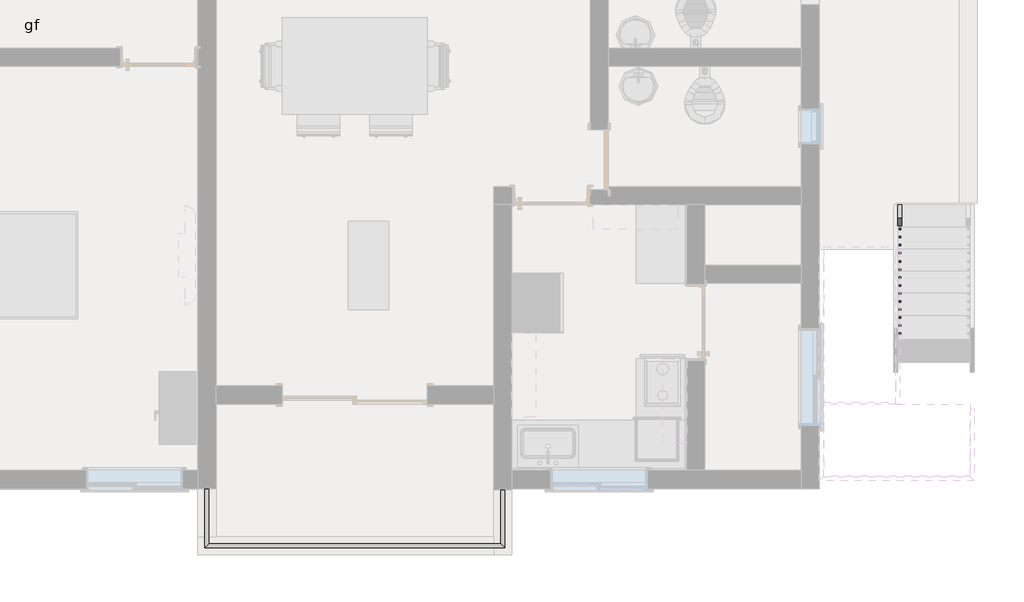
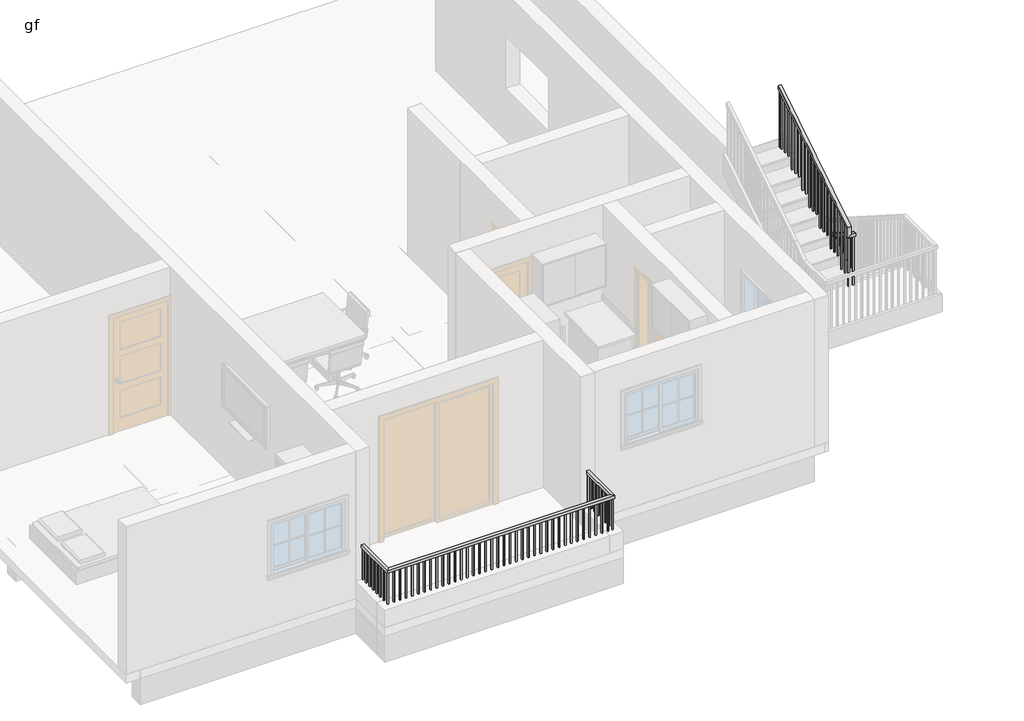
# One storey, part 4 of 8: 2 railings.
"""IFC4 building model written with IfcOpenShell, lengths in millimetres."""

from ifc_helpers import new_model, si_unit, frame, origin, place, context, project, spatial, polyline, outline, extrude, faceted_brep, element, save

model = new_model("IFC4")

# Units and contexts
model_context = context("Model", 3, world=origin())
ifc_project = project(units=[si_unit("LENGTHUNIT", "METRE", prefix="MILLI")], contexts=[model_context])

# Site, building, storey
site = spatial("IfcSite", under=ifc_project)
building = spatial("IfcBuilding", under=site)
storey = spatial("IfcBuildingStorey", under=building, Name="gf", Elevation=609.6)

# Railings
placement = place(None, origin())
element("IfcRailing", 1, ObjectType="Handrail - Rectangular", at=placement, inside=storey, context=model_context, shape_type="SolidModel", body=[
    faceted_brep([(-12350.8993763, -4611.6564015, 1524.0), (-12350.8993763, -4611.6564015, 1473.2), (-12401.6993763, -4611.6564015, 1473.2), (-12401.6993763, -4611.6564015, 1524.0), (-12350.8993763, -5303.8064015, 1524.0), (-12350.8993763, -5303.8064015, 1473.2), (-12401.6993763, -5354.6064015, 1473.2), (-12401.6993763, -5354.6064015, 1524.0), (-8667.8993763, -5303.8064015, 1524.0), (-8667.8993763, -5303.8064015, 1473.2), (-8617.0993763, -5354.6064015, 1473.2), (-8617.0993763, -5354.6064015, 1524.0), (-8667.8993763, -4618.0064015, 1524.0), (-8617.0993763, -4618.0064015, 1524.0), (-8617.0993763, -4618.0064015, 1473.2), (-8667.8993763, -4618.0064015, 1473.2)], [[[0, 1, 2, 3]], [[1, 0, 4, 5]], [[2, 1, 5, 6]], [[3, 2, 6, 7]], [[0, 3, 7, 4]], [[5, 4, 8, 9]], [[6, 5, 9, 10]], [[7, 6, 10, 11]], [[4, 7, 11, 8]], [[12, 13, 14, 15]], [[9, 8, 12, 15]], [[10, 9, 15, 14]], [[11, 10, 14, 13]], [[8, 11, 13, 12]]]),
    extrude(outline(polyline([(-8632.9743763, -4729.1314015), (-8652.0243763, -4729.1314015), (-8652.0243763, -4710.0814015), (-8632.9743763, -4710.0814015), (-8632.9743763, -4729.1314015)])), frame((0.0, 0.0, 609.6), z_axis=(0.0, 0.0, 1.0), x_axis=(1.0, 0.0, 0.0)), (0.0, 0.0, 1.0), 863.6),
    extrude(outline(polyline([(-8632.9743763, -4830.7314015), (-8652.0243763, -4830.7314015), (-8652.0243763, -4811.6814015), (-8632.9743763, -4811.6814015), (-8632.9743763, -4830.7314015)])), frame((0.0, 0.0, 609.6), z_axis=(0.0, 0.0, 1.0), x_axis=(1.0, 0.0, 0.0)), (0.0, 0.0, 1.0), 863.6),
    extrude(outline(polyline([(-8632.9743763, -4932.3314015), (-8652.0243763, -4932.3314015), (-8652.0243763, -4913.2814015), (-8632.9743763, -4913.2814015), (-8632.9743763, -4932.3314015)])), frame((0.0, 0.0, 609.6), z_axis=(0.0, 0.0, 1.0), x_axis=(1.0, 0.0, 0.0)), (0.0, 0.0, 1.0), 863.6),
    extrude(outline(polyline([(-8632.9743763, -5033.9314015), (-8652.0243763, -5033.9314015), (-8652.0243763, -5014.8814015), (-8632.9743763, -5014.8814015), (-8632.9743763, -5033.9314015)])), frame((0.0, 0.0, 609.6), z_axis=(0.0, 0.0, 1.0), x_axis=(1.0, 0.0, 0.0)), (0.0, 0.0, 1.0), 863.6),
    extrude(outline(polyline([(-8632.9743763, -5135.5314015), (-8652.0243763, -5135.5314015), (-8652.0243763, -5116.4814015), (-8632.9743763, -5116.4814015), (-8632.9743763, -5135.5314015)])), frame((0.0, 0.0, 609.6), z_axis=(0.0, 0.0, 1.0), x_axis=(1.0, 0.0, 0.0)), (0.0, 0.0, 1.0), 863.6),
    extrude(outline(polyline([(-8632.9743763, -5237.1314015), (-8652.0243763, -5237.1314015), (-8652.0243763, -5218.0814015), (-8632.9743763, -5218.0814015), (-8632.9743763, -5237.1314015)])), frame((0.0, 0.0, 609.6), z_axis=(0.0, 0.0, 1.0), x_axis=(1.0, 0.0, 0.0)), (0.0, 0.0, 1.0), 863.6),
    extrude(outline(polyline([(-8728.2243763, -5338.7314015), (-8728.2243763, -5319.6814015), (-8709.1743763, -5319.6814015), (-8709.1743763, -5338.7314015), (-8728.2243763, -5338.7314015)])), frame((0.0, 0.0, 609.6), z_axis=(0.0, 0.0, 1.0), x_axis=(1.0, 0.0, 0.0)), (0.0, 0.0, 1.0), 863.6),
    extrude(outline(polyline([(-8829.8243763, -5338.7314015), (-8829.8243763, -5319.6814015), (-8810.7743763, -5319.6814015), (-8810.7743763, -5338.7314015), (-8829.8243763, -5338.7314015)])), frame((0.0, 0.0, 609.6), z_axis=(0.0, 0.0, 1.0), x_axis=(1.0, 0.0, 0.0)), (0.0, 0.0, 1.0), 863.6),
    extrude(outline(polyline([(-8931.4243763, -5338.7314015), (-8931.4243763, -5319.6814015), (-8912.3743763, -5319.6814015), (-8912.3743763, -5338.7314015), (-8931.4243763, -5338.7314015)])), frame((0.0, 0.0, 609.6), z_axis=(0.0, 0.0, 1.0), x_axis=(1.0, 0.0, 0.0)), (0.0, 0.0, 1.0), 863.6),
    extrude(outline(polyline([(-9033.0243763, -5338.7314015), (-9033.0243763, -5319.6814015), (-9013.9743763, -5319.6814015), (-9013.9743763, -5338.7314015), (-9033.0243763, -5338.7314015)])), frame((0.0, 0.0, 609.6), z_axis=(0.0, 0.0, 1.0), x_axis=(1.0, 0.0, 0.0)), (0.0, 0.0, 1.0), 863.6),
    extrude(outline(polyline([(-9134.6243763, -5338.7314015), (-9134.6243763, -5319.6814015), (-9115.5743763, -5319.6814015), (-9115.5743763, -5338.7314015), (-9134.6243763, -5338.7314015)])), frame((0.0, 0.0, 609.6), z_axis=(0.0, 0.0, 1.0), x_axis=(1.0, 0.0, 0.0)), (0.0, 0.0, 1.0), 863.6),
    extrude(outline(polyline([(-9236.2243763, -5338.7314015), (-9236.2243763, -5319.6814015), (-9217.1743763, -5319.6814015), (-9217.1743763, -5338.7314015), (-9236.2243763, -5338.7314015)])), frame((0.0, 0.0, 609.6), z_axis=(0.0, 0.0, 1.0), x_axis=(1.0, 0.0, 0.0)), (0.0, 0.0, 1.0), 863.6),
    extrude(outline(polyline([(-9337.8243763, -5338.7314015), (-9337.8243763, -5319.6814015), (-9318.7743763, -5319.6814015), (-9318.7743763, -5338.7314015), (-9337.8243763, -5338.7314015)])), frame((0.0, 0.0, 609.6), z_axis=(0.0, 0.0, 1.0), x_axis=(1.0, 0.0, 0.0)), (0.0, 0.0, 1.0), 863.6),
    extrude(outline(polyline([(-9439.4243763, -5338.7314015), (-9439.4243763, -5319.6814015), (-9420.3743763, -5319.6814015), (-9420.3743763, -5338.7314015), (-9439.4243763, -5338.7314015)])), frame((0.0, 0.0, 609.6), z_axis=(0.0, 0.0, 1.0), x_axis=(1.0, 0.0, 0.0)), (0.0, 0.0, 1.0), 863.6),
    extrude(outline(polyline([(-9541.0243763, -5338.7314015), (-9541.0243763, -5319.6814015), (-9521.9743763, -5319.6814015), (-9521.9743763, -5338.7314015), (-9541.0243763, -5338.7314015)])), frame((0.0, 0.0, 609.6), z_axis=(0.0, 0.0, 1.0), x_axis=(1.0, 0.0, 0.0)), (0.0, 0.0, 1.0), 863.6),
    extrude(outline(polyline([(-9642.6243763, -5338.7314015), (-9642.6243763, -5319.6814015), (-9623.5743763, -5319.6814015), (-9623.5743763, -5338.7314015), (-9642.6243763, -5338.7314015)])), frame((0.0, 0.0, 609.6), z_axis=(0.0, 0.0, 1.0), x_axis=(1.0, 0.0, 0.0)), (0.0, 0.0, 1.0), 863.6),
    extrude(outline(polyline([(-9744.2243763, -5338.7314015), (-9744.2243763, -5319.6814015), (-9725.1743763, -5319.6814015), (-9725.1743763, -5338.7314015), (-9744.2243763, -5338.7314015)])), frame((0.0, 0.0, 609.6), z_axis=(0.0, 0.0, 1.0), x_axis=(1.0, 0.0, 0.0)), (0.0, 0.0, 1.0), 863.6),
    extrude(outline(polyline([(-9845.8243763, -5338.7314015), (-9845.8243763, -5319.6814015), (-9826.7743763, -5319.6814015), (-9826.7743763, -5338.7314015), (-9845.8243763, -5338.7314015)])), frame((0.0, 0.0, 609.6), z_axis=(0.0, 0.0, 1.0), x_axis=(1.0, 0.0, 0.0)), (0.0, 0.0, 1.0), 863.6),
    extrude(outline(polyline([(-9947.4243763, -5338.7314015), (-9947.4243763, -5319.6814015), (-9928.3743763, -5319.6814015), (-9928.3743763, -5338.7314015), (-9947.4243763, -5338.7314015)])), frame((0.0, 0.0, 609.6), z_axis=(0.0, 0.0, 1.0), x_axis=(1.0, 0.0, 0.0)), (0.0, 0.0, 1.0), 863.6),
    extrude(outline(polyline([(-10049.0243763, -5338.7314015), (-10049.0243763, -5319.6814015), (-10029.9743763, -5319.6814015), (-10029.9743763, -5338.7314015), (-10049.0243763, -5338.7314015)])), frame((0.0, 0.0, 609.6), z_axis=(0.0, 0.0, 1.0), x_axis=(1.0, 0.0, 0.0)), (0.0, 0.0, 1.0), 863.6),
    extrude(outline(polyline([(-10150.6243763, -5338.7314015), (-10150.6243763, -5319.6814015), (-10131.5743763, -5319.6814015), (-10131.5743763, -5338.7314015), (-10150.6243763, -5338.7314015)])), frame((0.0, 0.0, 609.6), z_axis=(0.0, 0.0, 1.0), x_axis=(1.0, 0.0, 0.0)), (0.0, 0.0, 1.0), 863.6),
    extrude(outline(polyline([(-10252.2243763, -5338.7314015), (-10252.2243763, -5319.6814015), (-10233.1743763, -5319.6814015), (-10233.1743763, -5338.7314015), (-10252.2243763, -5338.7314015)])), frame((0.0, 0.0, 609.6), z_axis=(0.0, 0.0, 1.0), x_axis=(1.0, 0.0, 0.0)), (0.0, 0.0, 1.0), 863.6),
    extrude(outline(polyline([(-10353.8243763, -5338.7314015), (-10353.8243763, -5319.6814015), (-10334.7743763, -5319.6814015), (-10334.7743763, -5338.7314015), (-10353.8243763, -5338.7314015)])), frame((0.0, 0.0, 609.6), z_axis=(0.0, 0.0, 1.0), x_axis=(1.0, 0.0, 0.0)), (0.0, 0.0, 1.0), 863.6),
    extrude(outline(polyline([(-10455.4243763, -5338.7314015), (-10455.4243763, -5319.6814015), (-10436.3743763, -5319.6814015), (-10436.3743763, -5338.7314015), (-10455.4243763, -5338.7314015)])), frame((0.0, 0.0, 609.6), z_axis=(0.0, 0.0, 1.0), x_axis=(1.0, 0.0, 0.0)), (0.0, 0.0, 1.0), 863.6),
    extrude(outline(polyline([(-10557.0243763, -5338.7314015), (-10557.0243763, -5319.6814015), (-10537.9743763, -5319.6814015), (-10537.9743763, -5338.7314015), (-10557.0243763, -5338.7314015)])), frame((0.0, 0.0, 609.6), z_axis=(0.0, 0.0, 1.0), x_axis=(1.0, 0.0, 0.0)), (0.0, 0.0, 1.0), 863.6),
    extrude(outline(polyline([(-10658.6243763, -5338.7314015), (-10658.6243763, -5319.6814015), (-10639.5743763, -5319.6814015), (-10639.5743763, -5338.7314015), (-10658.6243763, -5338.7314015)])), frame((0.0, 0.0, 609.6), z_axis=(0.0, 0.0, 1.0), x_axis=(1.0, 0.0, 0.0)), (0.0, 0.0, 1.0), 863.6),
    extrude(outline(polyline([(-10760.2243763, -5338.7314015), (-10760.2243763, -5319.6814015), (-10741.1743763, -5319.6814015), (-10741.1743763, -5338.7314015), (-10760.2243763, -5338.7314015)])), frame((0.0, 0.0, 609.6), z_axis=(0.0, 0.0, 1.0), x_axis=(1.0, 0.0, 0.0)), (0.0, 0.0, 1.0), 863.6),
    extrude(outline(polyline([(-10861.8243763, -5338.7314015), (-10861.8243763, -5319.6814015), (-10842.7743763, -5319.6814015), (-10842.7743763, -5338.7314015), (-10861.8243763, -5338.7314015)])), frame((0.0, 0.0, 609.6), z_axis=(0.0, 0.0, 1.0), x_axis=(1.0, 0.0, 0.0)), (0.0, 0.0, 1.0), 863.6),
    extrude(outline(polyline([(-10963.4243763, -5338.7314015), (-10963.4243763, -5319.6814015), (-10944.3743763, -5319.6814015), (-10944.3743763, -5338.7314015), (-10963.4243763, -5338.7314015)])), frame((0.0, 0.0, 609.6), z_axis=(0.0, 0.0, 1.0), x_axis=(1.0, 0.0, 0.0)), (0.0, 0.0, 1.0), 863.6),
    extrude(outline(polyline([(-11065.0243763, -5338.7314015), (-11065.0243763, -5319.6814015), (-11045.9743763, -5319.6814015), (-11045.9743763, -5338.7314015), (-11065.0243763, -5338.7314015)])), frame((0.0, 0.0, 609.6), z_axis=(0.0, 0.0, 1.0), x_axis=(1.0, 0.0, 0.0)), (0.0, 0.0, 1.0), 863.6),
    extrude(outline(polyline([(-11166.6243763, -5338.7314015), (-11166.6243763, -5319.6814015), (-11147.5743763, -5319.6814015), (-11147.5743763, -5338.7314015), (-11166.6243763, -5338.7314015)])), frame((0.0, 0.0, 609.6), z_axis=(0.0, 0.0, 1.0), x_axis=(1.0, 0.0, 0.0)), (0.0, 0.0, 1.0), 863.6),
    extrude(outline(polyline([(-11268.2243763, -5338.7314015), (-11268.2243763, -5319.6814015), (-11249.1743763, -5319.6814015), (-11249.1743763, -5338.7314015), (-11268.2243763, -5338.7314015)])), frame((0.0, 0.0, 609.6), z_axis=(0.0, 0.0, 1.0), x_axis=(1.0, 0.0, 0.0)), (0.0, 0.0, 1.0), 863.6),
    extrude(outline(polyline([(-11369.8243763, -5338.7314015), (-11369.8243763, -5319.6814015), (-11350.7743763, -5319.6814015), (-11350.7743763, -5338.7314015), (-11369.8243763, -5338.7314015)])), frame((0.0, 0.0, 609.6), z_axis=(0.0, 0.0, 1.0), x_axis=(1.0, 0.0, 0.0)), (0.0, 0.0, 1.0), 863.6),
    extrude(outline(polyline([(-11471.4243763, -5338.7314015), (-11471.4243763, -5319.6814015), (-11452.3743763, -5319.6814015), (-11452.3743763, -5338.7314015), (-11471.4243763, -5338.7314015)])), frame((0.0, 0.0, 609.6), z_axis=(0.0, 0.0, 1.0), x_axis=(1.0, 0.0, 0.0)), (0.0, 0.0, 1.0), 863.6),
    extrude(outline(polyline([(-11573.0243763, -5338.7314015), (-11573.0243763, -5319.6814015), (-11553.9743763, -5319.6814015), (-11553.9743763, -5338.7314015), (-11573.0243763, -5338.7314015)])), frame((0.0, 0.0, 609.6), z_axis=(0.0, 0.0, 1.0), x_axis=(1.0, 0.0, 0.0)), (0.0, 0.0, 1.0), 863.6),
    extrude(outline(polyline([(-11674.6243763, -5338.7314015), (-11674.6243763, -5319.6814015), (-11655.5743763, -5319.6814015), (-11655.5743763, -5338.7314015), (-11674.6243763, -5338.7314015)])), frame((0.0, 0.0, 609.6), z_axis=(0.0, 0.0, 1.0), x_axis=(1.0, 0.0, 0.0)), (0.0, 0.0, 1.0), 863.6),
    extrude(outline(polyline([(-11776.2243763, -5338.7314015), (-11776.2243763, -5319.6814015), (-11757.1743763, -5319.6814015), (-11757.1743763, -5338.7314015), (-11776.2243763, -5338.7314015)])), frame((0.0, 0.0, 609.6), z_axis=(0.0, 0.0, 1.0), x_axis=(1.0, 0.0, 0.0)), (0.0, 0.0, 1.0), 863.6),
    extrude(outline(polyline([(-11877.8243763, -5338.7314015), (-11877.8243763, -5319.6814015), (-11858.7743763, -5319.6814015), (-11858.7743763, -5338.7314015), (-11877.8243763, -5338.7314015)])), frame((0.0, 0.0, 609.6), z_axis=(0.0, 0.0, 1.0), x_axis=(1.0, 0.0, 0.0)), (0.0, 0.0, 1.0), 863.6),
    extrude(outline(polyline([(-11979.4243763, -5338.7314015), (-11979.4243763, -5319.6814015), (-11960.3743763, -5319.6814015), (-11960.3743763, -5338.7314015), (-11979.4243763, -5338.7314015)])), frame((0.0, 0.0, 609.6), z_axis=(0.0, 0.0, 1.0), x_axis=(1.0, 0.0, 0.0)), (0.0, 0.0, 1.0), 863.6),
    extrude(outline(polyline([(-12081.0243763, -5338.7314015), (-12081.0243763, -5319.6814015), (-12061.9743763, -5319.6814015), (-12061.9743763, -5338.7314015), (-12081.0243763, -5338.7314015)])), frame((0.0, 0.0, 609.6), z_axis=(0.0, 0.0, 1.0), x_axis=(1.0, 0.0, 0.0)), (0.0, 0.0, 1.0), 863.6),
    extrude(outline(polyline([(-12182.6243763, -5338.7314015), (-12182.6243763, -5319.6814015), (-12163.5743763, -5319.6814015), (-12163.5743763, -5338.7314015), (-12182.6243763, -5338.7314015)])), frame((0.0, 0.0, 609.6), z_axis=(0.0, 0.0, 1.0), x_axis=(1.0, 0.0, 0.0)), (0.0, 0.0, 1.0), 863.6),
    extrude(outline(polyline([(-12284.2243763, -5338.7314015), (-12284.2243763, -5319.6814015), (-12265.1743763, -5319.6814015), (-12265.1743763, -5338.7314015), (-12284.2243763, -5338.7314015)])), frame((0.0, 0.0, 609.6), z_axis=(0.0, 0.0, 1.0), x_axis=(1.0, 0.0, 0.0)), (0.0, 0.0, 1.0), 863.6),
    extrude(outline(polyline([(-12385.8243763, -5313.3314015), (-12366.7743763, -5313.3314015), (-12366.7743763, -5332.3814015), (-12385.8243763, -5332.3814015), (-12385.8243763, -5313.3314015)])), frame((0.0, 0.0, 609.6), z_axis=(0.0, 0.0, 1.0), x_axis=(1.0, 0.0, 0.0)), (0.0, 0.0, 1.0), 863.6),
    extrude(outline(polyline([(-12385.8243763, -5211.7314015), (-12366.7743763, -5211.7314015), (-12366.7743763, -5230.7814015), (-12385.8243763, -5230.7814015), (-12385.8243763, -5211.7314015)])), frame((0.0, 0.0, 609.6), z_axis=(0.0, 0.0, 1.0), x_axis=(1.0, 0.0, 0.0)), (0.0, 0.0, 1.0), 863.6),
    extrude(outline(polyline([(-12385.8243763, -5110.1314015), (-12366.7743763, -5110.1314015), (-12366.7743763, -5129.1814015), (-12385.8243763, -5129.1814015), (-12385.8243763, -5110.1314015)])), frame((0.0, 0.0, 609.6), z_axis=(0.0, 0.0, 1.0), x_axis=(1.0, 0.0, 0.0)), (0.0, 0.0, 1.0), 863.6),
    extrude(outline(polyline([(-12385.8243763, -5008.5314015), (-12366.7743763, -5008.5314015), (-12366.7743763, -5027.5814015), (-12385.8243763, -5027.5814015), (-12385.8243763, -5008.5314015)])), frame((0.0, 0.0, 609.6), z_axis=(0.0, 0.0, 1.0), x_axis=(1.0, 0.0, 0.0)), (0.0, 0.0, 1.0), 863.6),
    extrude(outline(polyline([(-12385.8243763, -4906.9314015), (-12366.7743763, -4906.9314015), (-12366.7743763, -4925.9814015), (-12385.8243763, -4925.9814015), (-12385.8243763, -4906.9314015)])), frame((0.0, 0.0, 609.6), z_axis=(0.0, 0.0, 1.0), x_axis=(1.0, 0.0, 0.0)), (0.0, 0.0, 1.0), 863.6),
    extrude(outline(polyline([(-12385.8243763, -4805.3314015), (-12366.7743763, -4805.3314015), (-12366.7743763, -4824.3814015), (-12385.8243763, -4824.3814015), (-12385.8243763, -4805.3314015)])), frame((0.0, 0.0, 609.6), z_axis=(0.0, 0.0, 1.0), x_axis=(1.0, 0.0, 0.0)), (0.0, 0.0, 1.0), 863.6),
    extrude(outline(polyline([(-12385.8243763, -4703.7314015), (-12366.7743763, -4703.7314015), (-12366.7743763, -4722.7814015), (-12385.8243763, -4722.7814015), (-12385.8243763, -4703.7314015)])), frame((0.0, 0.0, 609.6), z_axis=(0.0, 0.0, 1.0), x_axis=(1.0, 0.0, 0.0)), (0.0, 0.0, 1.0), 863.6),
    extrude(outline(polyline([(-8652.0243763, -5338.7314015), (-8652.0243763, -5319.6814015), (-8632.9743763, -5319.6814015), (-8632.9743763, -5338.7314015), (-8652.0243763, -5338.7314015)])), frame((0.0, 0.0, 609.6), z_axis=(0.0, 0.0, 1.0), x_axis=(1.0, 0.0, 0.0)), (0.0, 0.0, 1.0), 863.6),
    extrude(outline(polyline([(-12385.8243763, -5319.6814015), (-12366.7743763, -5319.6814015), (-12366.7743763, -5338.7314015), (-12385.8243763, -5338.7314015), (-12385.8243763, -5319.6814015)])), frame((0.0, 0.0, 609.6), z_axis=(0.0, 0.0, 1.0), x_axis=(1.0, 0.0, 0.0)), (0.0, 0.0, 1.0), 863.6),
    extrude(outline(polyline([(-8632.9743763, -4637.0564015), (-8652.0243763, -4637.0564015), (-8652.0243763, -4618.0064015), (-8632.9743763, -4618.0064015), (-8632.9743763, -4637.0564015)])), frame((0.0, 0.0, 609.6), z_axis=(0.0, 0.0, 1.0), x_axis=(1.0, 0.0, 0.0)), (0.0, 0.0, 1.0), 863.6),
    extrude(outline(polyline([(-12385.8243763, -4611.6564015), (-12366.7743763, -4611.6564015), (-12366.7743763, -4630.7064015), (-12385.8243763, -4630.7064015), (-12385.8243763, -4611.6564015)])), frame((0.0, 0.0, 609.6), z_axis=(0.0, 0.0, 1.0), x_axis=(1.0, 0.0, 0.0)), (0.0, 0.0, 1.0), 863.6),
])
element("IfcRailing", 2, ObjectType="Handrail - Rectangular", at=placement, inside=storey, context=model_context, shape_type="SolidModel", body=[
    faceted_brep([(-3600.5993763, -1023.9064015, 1701.8), (-3600.5993763, -1023.9064015, 1641.586276), (-3651.3993763, -1023.9064015, 1641.586276), (-3651.3993763, -1023.9064015, 1701.8), (-3600.5993763, -3538.5064015, 3302.0), (-3651.3993763, -3538.5064015, 3302.0), (-3651.3993763, -3538.5064015, 3241.786276), (-3600.5993763, -3538.5064015, 3241.786276)], [[[0, 1, 2, 3]], [[4, 5, 6, 7]], [[1, 0, 4, 7]], [[2, 1, 7, 6]], [[3, 2, 6, 5]], [[0, 3, 5, 4]]]),
    faceted_brep([(-3600.5993763, -3589.3064015, 3302.0), (-3600.5993763, -3589.3064015, 3251.2), (-3600.5993763, -3538.5064015, 3251.2), (-3600.5993763, -3538.5064015, 3302.0), (-3676.7993763, -3589.3064015, 3302.0), (-3676.7993763, -3538.5064015, 3302.0), (-3727.5993763, -3538.5064015, 3251.2), (-3727.5993763, -3589.3064015, 3251.2)], [[[0, 1, 2, 3]], [[4, 5, 6, 7]], [[1, 0, 4, 7]], [[2, 1, 7, 6]], [[3, 2, 6, 5]], [[0, 3, 5, 4]]]),
    faceted_brep([(-3676.7993763, -3589.3064015, 3302.0), (-3727.5993763, -3589.3064015, 3251.2), (-3727.5993763, -3538.5064015, 3251.2), (-3676.7993763, -3538.5064015, 3302.0), (-3676.7993763, -3589.3064015, 3447.4727273), (-3676.7993763, -3538.5064015, 3419.586276), (-3727.5993763, -3538.5064015, 3419.586276), (-3727.5993763, -3589.3064015, 3447.4727273)], [[[0, 1, 2, 3]], [[4, 5, 6, 7]], [[1, 0, 4, 7]], [[2, 1, 7, 6]], [[3, 2, 6, 5]], [[0, 3, 5, 4]]]),
    faceted_brep([(-3727.5993763, -3589.3064015, 3447.4727273), (-3727.5993763, -3538.5064015, 3419.586276), (-3676.7993763, -3538.5064015, 3419.586276), (-3676.7993763, -3589.3064015, 3447.4727273), (-3727.5993763, -1582.7064015, 4724.4), (-3676.7993763, -1582.7064015, 4724.4), (-3676.7993763, -1582.7064015, 4664.186276), (-3727.5993763, -1582.7064015, 4664.186276)], [[[0, 1, 2, 3]], [[4, 5, 6, 7]], [[1, 0, 4, 7]], [[2, 1, 7, 6]], [[3, 2, 6, 5]], [[0, 3, 5, 4]]]),
    extrude(outline(polyline([(-1643.0314015, 4625.7976396), (-1623.9814015, 4637.9203669), (-1623.9814015, 3632.2), (-1643.0314015, 3632.2), (-1643.0314015, 4625.7976396)])), frame((-3711.7243763, 0.0, 0.0), z_axis=(1.0, 0.0, 0.0), x_axis=(0.0, 1.0, 0.0)), (0.0, 0.0, 1.0), 19.05),
    extrude(outline(polyline([(-1744.6314015, 4561.1430941), (-1725.5814015, 4573.2658214), (-1725.5814015, 3632.2), (-1744.6314015, 3632.2), (-1744.6314015, 4561.1430941)])), frame((-3711.7243763, 0.0, 0.0), z_axis=(1.0, 0.0, 0.0), x_axis=(0.0, 1.0, 0.0)), (0.0, 0.0, 1.0), 19.05),
    extrude(outline(polyline([(-1846.2314015, 4496.4885487), (-1827.1814015, 4508.611276), (-1827.1814015, 3632.2), (-1846.2314015, 3632.2), (-1846.2314015, 4496.4885487)])), frame((-3711.7243763, 0.0, 0.0), z_axis=(1.0, 0.0, 0.0), x_axis=(0.0, 1.0, 0.0)), (0.0, 0.0, 1.0), 19.05),
    extrude(outline(polyline([(-1947.8314015, 4431.8340032), (-1928.7814015, 4443.9567305), (-1928.7814015, 3454.4), (-1947.8314015, 3454.4), (-1947.8314015, 4431.8340032)])), frame((-3711.7243763, 0.0, 0.0), z_axis=(1.0, 0.0, 0.0), x_axis=(0.0, 1.0, 0.0)), (0.0, 0.0, 1.0), 19.05),
    extrude(outline(polyline([(-2049.4314015, 4367.1794578), (-2030.3814015, 4379.3021851), (-2030.3814015, 3454.4), (-2049.4314015, 3454.4), (-2049.4314015, 4367.1794578)])), frame((-3711.7243763, 0.0, 0.0), z_axis=(1.0, 0.0, 0.0), x_axis=(0.0, 1.0, 0.0)), (0.0, 0.0, 1.0), 19.05),
    extrude(outline(polyline([(-2151.0314015, 4302.5249123), (-2131.9814015, 4314.6476396), (-2131.9814015, 3454.4), (-2151.0314015, 3454.4), (-2151.0314015, 4302.5249123)])), frame((-3711.7243763, 0.0, 0.0), z_axis=(1.0, 0.0, 0.0), x_axis=(0.0, 1.0, 0.0)), (0.0, 0.0, 1.0), 19.05),
    extrude(outline(polyline([(-2252.6314015, 4237.8703669), (-2233.5814015, 4249.9930941), (-2233.5814015, 3276.6), (-2252.6314015, 3276.6), (-2252.6314015, 4237.8703669)])), frame((-3711.7243763, 0.0, 0.0), z_axis=(1.0, 0.0, 0.0), x_axis=(0.0, 1.0, 0.0)), (0.0, 0.0, 1.0), 19.05),
    extrude(outline(polyline([(-2354.2314015, 4173.2158214), (-2335.1814015, 4185.3385487), (-2335.1814015, 3276.6), (-2354.2314015, 3276.6), (-2354.2314015, 4173.2158214)])), frame((-3711.7243763, 0.0, 0.0), z_axis=(1.0, 0.0, 0.0), x_axis=(0.0, 1.0, 0.0)), (0.0, 0.0, 1.0), 19.05),
    extrude(outline(polyline([(-2455.8314015, 4108.561276), (-2436.7814015, 4120.6840032), (-2436.7814015, 3098.8), (-2455.8314015, 3098.8), (-2455.8314015, 4108.561276)])), frame((-3711.7243763, 0.0, 0.0), z_axis=(1.0, 0.0, 0.0), x_axis=(0.0, 1.0, 0.0)), (0.0, 0.0, 1.0), 19.05),
    extrude(outline(polyline([(-2557.4314015, 4043.9067305), (-2538.3814015, 4056.0294578), (-2538.3814015, 3098.8), (-2557.4314015, 3098.8), (-2557.4314015, 4043.9067305)])), frame((-3711.7243763, 0.0, 0.0), z_axis=(1.0, 0.0, 0.0), x_axis=(0.0, 1.0, 0.0)), (0.0, 0.0, 1.0), 19.05),
    extrude(outline(polyline([(-2659.0314015, 3979.2521851), (-2639.9814015, 3991.3749123), (-2639.9814015, 3098.8), (-2659.0314015, 3098.8), (-2659.0314015, 3979.2521851)])), frame((-3711.7243763, 0.0, 0.0), z_axis=(1.0, 0.0, 0.0), x_axis=(0.0, 1.0, 0.0)), (0.0, 0.0, 1.0), 19.05),
    extrude(outline(polyline([(-2760.6314015, 3914.5976396), (-2741.5814015, 3926.7203669), (-2741.5814015, 2921.0), (-2760.6314015, 2921.0), (-2760.6314015, 3914.5976396)])), frame((-3711.7243763, 0.0, 0.0), z_axis=(1.0, 0.0, 0.0), x_axis=(0.0, 1.0, 0.0)), (0.0, 0.0, 1.0), 19.05),
    extrude(outline(polyline([(-2862.2314015, 3849.9430941), (-2843.1814015, 3862.0658214), (-2843.1814015, 2921.0), (-2862.2314015, 2921.0), (-2862.2314015, 3849.9430941)])), frame((-3711.7243763, 0.0, 0.0), z_axis=(1.0, 0.0, 0.0), x_axis=(0.0, 1.0, 0.0)), (0.0, 0.0, 1.0), 19.05),
    extrude(outline(polyline([(-2963.8314015, 3785.2885487), (-2944.7814015, 3797.411276), (-2944.7814015, 2921.0), (-2963.8314015, 2921.0), (-2963.8314015, 3785.2885487)])), frame((-3711.7243763, 0.0, 0.0), z_axis=(1.0, 0.0, 0.0), x_axis=(0.0, 1.0, 0.0)), (0.0, 0.0, 1.0), 19.05),
    extrude(outline(polyline([(-3065.4314015, 3720.6340032), (-3046.3814015, 3732.7567305), (-3046.3814015, 2743.2), (-3065.4314015, 2743.2), (-3065.4314015, 3720.6340032)])), frame((-3711.7243763, 0.0, 0.0), z_axis=(1.0, 0.0, 0.0), x_axis=(0.0, 1.0, 0.0)), (0.0, 0.0, 1.0), 19.05),
    extrude(outline(polyline([(-3167.0314015, 3655.9794578), (-3147.9814015, 3668.1021851), (-3147.9814015, 2743.2), (-3167.0314015, 2743.2), (-3167.0314015, 3655.9794578)])), frame((-3711.7243763, 0.0, 0.0), z_axis=(1.0, 0.0, 0.0), x_axis=(0.0, 1.0, 0.0)), (0.0, 0.0, 1.0), 19.05),
    extrude(outline(polyline([(-3268.6314015, 3591.3249123), (-3249.5814015, 3603.4476396), (-3249.5814015, 2743.2), (-3268.6314015, 2743.2), (-3268.6314015, 3591.3249123)])), frame((-3711.7243763, 0.0, 0.0), z_axis=(1.0, 0.0, 0.0), x_axis=(0.0, 1.0, 0.0)), (0.0, 0.0, 1.0), 19.05),
    extrude(outline(polyline([(-3370.2314015, 3526.6703669), (-3351.1814015, 3538.7930941), (-3351.1814015, 2565.4), (-3370.2314015, 2565.4), (-3370.2314015, 3526.6703669)])), frame((-3711.7243763, 0.0, 0.0), z_axis=(1.0, 0.0, 0.0), x_axis=(0.0, 1.0, 0.0)), (0.0, 0.0, 1.0), 19.05),
    extrude(outline(polyline([(-3471.8314015, 3462.0158214), (-3452.7814015, 3474.1385487), (-3452.7814015, 2565.4), (-3471.8314015, 2565.4), (-3471.8314015, 3462.0158214)])), frame((-3711.7243763, 0.0, 0.0), z_axis=(1.0, 0.0, 0.0), x_axis=(0.0, 1.0, 0.0)), (0.0, 0.0, 1.0), 19.05),
    extrude(outline(polyline([(-3471.8314015, 3199.3567305), (-3452.7814015, 3187.2340032), (-3452.7814015, 2209.8), (-3471.8314015, 2209.8), (-3471.8314015, 3199.3567305)])), frame((-3635.5243763, 0.0, 0.0), z_axis=(1.0, 0.0, 0.0), x_axis=(0.0, 1.0, 0.0)), (0.0, 0.0, 1.0), 19.05),
    extrude(outline(polyline([(-3370.2314015, 3134.7021851), (-3351.1814015, 3122.5794578), (-3351.1814015, 2209.8), (-3370.2314015, 2209.8), (-3370.2314015, 3134.7021851)])), frame((-3635.5243763, 0.0, 0.0), z_axis=(1.0, 0.0, 0.0), x_axis=(0.0, 1.0, 0.0)), (0.0, 0.0, 1.0), 19.05),
    extrude(outline(polyline([(-3268.6314015, 3070.0476396), (-3249.5814015, 3057.9249123), (-3249.5814015, 2209.8), (-3268.6314015, 2209.8), (-3268.6314015, 3070.0476396)])), frame((-3635.5243763, 0.0, 0.0), z_axis=(1.0, 0.0, 0.0), x_axis=(0.0, 1.0, 0.0)), (0.0, 0.0, 1.0), 19.05),
    extrude(outline(polyline([(-3167.0314015, 3005.3930941), (-3147.9814015, 2993.2703669), (-3147.9814015, 2032.0), (-3167.0314015, 2032.0), (-3167.0314015, 3005.3930941)])), frame((-3635.5243763, 0.0, 0.0), z_axis=(1.0, 0.0, 0.0), x_axis=(0.0, 1.0, 0.0)), (0.0, 0.0, 1.0), 19.05),
    extrude(outline(polyline([(-3065.4314015, 2940.7385487), (-3046.3814015, 2928.6158214), (-3046.3814015, 2032.0), (-3065.4314015, 2032.0), (-3065.4314015, 2940.7385487)])), frame((-3635.5243763, 0.0, 0.0), z_axis=(1.0, 0.0, 0.0), x_axis=(0.0, 1.0, 0.0)), (0.0, 0.0, 1.0), 19.05),
    extrude(outline(polyline([(-2963.8314015, 2876.0840032), (-2944.7814015, 2863.961276), (-2944.7814015, 1854.2), (-2963.8314015, 1854.2), (-2963.8314015, 2876.0840032)])), frame((-3635.5243763, 0.0, 0.0), z_axis=(1.0, 0.0, 0.0), x_axis=(0.0, 1.0, 0.0)), (0.0, 0.0, 1.0), 19.05),
    extrude(outline(polyline([(-2862.2314015, 2811.4294578), (-2843.1814015, 2799.3067305), (-2843.1814015, 1854.2), (-2862.2314015, 1854.2), (-2862.2314015, 2811.4294578)])), frame((-3635.5243763, 0.0, 0.0), z_axis=(1.0, 0.0, 0.0), x_axis=(0.0, 1.0, 0.0)), (0.0, 0.0, 1.0), 19.05),
    extrude(outline(polyline([(-2760.6314015, 2746.7749123), (-2741.5814015, 2734.6521851), (-2741.5814015, 1854.2), (-2760.6314015, 1854.2), (-2760.6314015, 2746.7749123)])), frame((-3635.5243763, 0.0, 0.0), z_axis=(1.0, 0.0, 0.0), x_axis=(0.0, 1.0, 0.0)), (0.0, 0.0, 1.0), 19.05),
    extrude(outline(polyline([(-2659.0314015, 2682.1203669), (-2639.9814015, 2669.9976396), (-2639.9814015, 1676.4), (-2659.0314015, 1676.4), (-2659.0314015, 2682.1203669)])), frame((-3635.5243763, 0.0, 0.0), z_axis=(1.0, 0.0, 0.0), x_axis=(0.0, 1.0, 0.0)), (0.0, 0.0, 1.0), 19.05),
    extrude(outline(polyline([(-2557.4314015, 2617.4658214), (-2538.3814015, 2605.3430941), (-2538.3814015, 1676.4), (-2557.4314015, 1676.4), (-2557.4314015, 2617.4658214)])), frame((-3635.5243763, 0.0, 0.0), z_axis=(1.0, 0.0, 0.0), x_axis=(0.0, 1.0, 0.0)), (0.0, 0.0, 1.0), 19.05),
    extrude(outline(polyline([(-2455.8314015, 2552.811276), (-2436.7814015, 2540.6885487), (-2436.7814015, 1676.4), (-2455.8314015, 1676.4), (-2455.8314015, 2552.811276)])), frame((-3635.5243763, 0.0, 0.0), z_axis=(1.0, 0.0, 0.0), x_axis=(0.0, 1.0, 0.0)), (0.0, 0.0, 1.0), 19.05),
    extrude(outline(polyline([(-2354.2314015, 2488.1567305), (-2335.1814015, 2476.0340032), (-2335.1814015, 1498.6), (-2354.2314015, 1498.6), (-2354.2314015, 2488.1567305)])), frame((-3635.5243763, 0.0, 0.0), z_axis=(1.0, 0.0, 0.0), x_axis=(0.0, 1.0, 0.0)), (0.0, 0.0, 1.0), 19.05),
    extrude(outline(polyline([(-2252.6314015, 2423.5021851), (-2233.5814015, 2411.3794578), (-2233.5814015, 1498.6), (-2252.6314015, 1498.6), (-2252.6314015, 2423.5021851)])), frame((-3635.5243763, 0.0, 0.0), z_axis=(1.0, 0.0, 0.0), x_axis=(0.0, 1.0, 0.0)), (0.0, 0.0, 1.0), 19.05),
    extrude(outline(polyline([(-2151.0314015, 2358.8476396), (-2131.9814015, 2346.7249123), (-2131.9814015, 1498.6), (-2151.0314015, 1498.6), (-2151.0314015, 2358.8476396)])), frame((-3635.5243763, 0.0, 0.0), z_axis=(1.0, 0.0, 0.0), x_axis=(0.0, 1.0, 0.0)), (0.0, 0.0, 1.0), 19.05),
    extrude(outline(polyline([(-2049.4314015, 2294.1930941), (-2030.3814015, 2282.0703669), (-2030.3814015, 1320.8), (-2049.4314015, 1320.8), (-2049.4314015, 2294.1930941)])), frame((-3635.5243763, 0.0, 0.0), z_axis=(1.0, 0.0, 0.0), x_axis=(0.0, 1.0, 0.0)), (0.0, 0.0, 1.0), 19.05),
    extrude(outline(polyline([(-1947.8314015, 2229.5385487), (-1928.7814015, 2217.4158214), (-1928.7814015, 1320.8), (-1947.8314015, 1320.8), (-1947.8314015, 2229.5385487)])), frame((-3635.5243763, 0.0, 0.0), z_axis=(1.0, 0.0, 0.0), x_axis=(0.0, 1.0, 0.0)), (0.0, 0.0, 1.0), 19.05),
    extrude(outline(polyline([(-1846.2314015, 2164.8840032), (-1827.1814015, 2152.761276), (-1827.1814015, 1143.0), (-1846.2314015, 1143.0), (-1846.2314015, 2164.8840032)])), frame((-3635.5243763, 0.0, 0.0), z_axis=(1.0, 0.0, 0.0), x_axis=(0.0, 1.0, 0.0)), (0.0, 0.0, 1.0), 19.05),
    extrude(outline(polyline([(-1744.6314015, 2100.2294578), (-1725.5814015, 2088.1067305), (-1725.5814015, 1143.0), (-1744.6314015, 1143.0), (-1744.6314015, 2100.2294578)])), frame((-3635.5243763, 0.0, 0.0), z_axis=(1.0, 0.0, 0.0), x_axis=(0.0, 1.0, 0.0)), (0.0, 0.0, 1.0), 19.05),
    extrude(outline(polyline([(-1643.0314015, 2035.5749123), (-1623.9814015, 2023.4521851), (-1623.9814015, 1143.0), (-1643.0314015, 1143.0), (-1643.0314015, 2035.5749123)])), frame((-3635.5243763, 0.0, 0.0), z_axis=(1.0, 0.0, 0.0), x_axis=(0.0, 1.0, 0.0)), (0.0, 0.0, 1.0), 19.05),
    extrude(outline(polyline([(-1541.4314015, 1970.9203669), (-1522.3814015, 1958.7976396), (-1522.3814015, 965.2), (-1541.4314015, 965.2), (-1541.4314015, 1970.9203669)])), frame((-3635.5243763, 0.0, 0.0), z_axis=(1.0, 0.0, 0.0), x_axis=(0.0, 1.0, 0.0)), (0.0, 0.0, 1.0), 19.05),
    extrude(outline(polyline([(-1439.8314015, 1906.2658214), (-1420.7814015, 1894.1430941), (-1420.7814015, 965.2), (-1439.8314015, 965.2), (-1439.8314015, 1906.2658214)])), frame((-3635.5243763, 0.0, 0.0), z_axis=(1.0, 0.0, 0.0), x_axis=(0.0, 1.0, 0.0)), (0.0, 0.0, 1.0), 19.05),
    extrude(outline(polyline([(-1338.2314015, 1841.611276), (-1319.1814015, 1829.4885487), (-1319.1814015, 965.2), (-1338.2314015, 965.2), (-1338.2314015, 1841.611276)])), frame((-3635.5243763, 0.0, 0.0), z_axis=(1.0, 0.0, 0.0), x_axis=(0.0, 1.0, 0.0)), (0.0, 0.0, 1.0), 19.05),
    extrude(outline(polyline([(-1236.6314015, 1776.9567305), (-1217.5814015, 1764.8340032), (-1217.5814015, 787.4), (-1236.6314015, 787.4), (-1236.6314015, 1776.9567305)])), frame((-3635.5243763, 0.0, 0.0), z_axis=(1.0, 0.0, 0.0), x_axis=(0.0, 1.0, 0.0)), (0.0, 0.0, 1.0), 19.05),
    extrude(outline(polyline([(-1135.0314015, 1712.3021851), (-1115.9814015, 1700.1794578), (-1115.9814015, 787.4), (-1135.0314015, 787.4), (-1135.0314015, 1712.3021851)])), frame((-3635.5243763, 0.0, 0.0), z_axis=(1.0, 0.0, 0.0), x_axis=(0.0, 1.0, 0.0)), (0.0, 0.0, 1.0), 19.05),
    extrude(outline(polyline([(-3692.6743763, -3554.3814015), (-3692.6743763, -3573.4314015), (-3711.7243763, -3573.4314015), (-3711.7243763, -3554.3814015), (-3692.6743763, -3554.3814015)])), frame((0.0, 0.0, 2387.6), z_axis=(0.0, 0.0, 1.0), x_axis=(1.0, 0.0, 0.0)), (0.0, 0.0, 1.0), 863.6),
    extrude(outline(polyline([(-3573.4314015, 3264.011276), (-3554.3814015, 3251.8885487), (-3554.3814015, 2387.6), (-3573.4314015, 2387.6), (-3573.4314015, 3264.011276)])), frame((-3635.5243763, 0.0, 0.0), z_axis=(1.0, 0.0, 0.0), x_axis=(0.0, 1.0, 0.0)), (0.0, 0.0, 1.0), 19.05),
    extrude(outline(polyline([(-1601.7564015, 4652.0635487), (-1582.7064015, 4664.186276), (-1582.7064015, 3632.2), (-1601.7564015, 3632.2), (-1601.7564015, 4652.0635487)])), frame((-3711.7243763, 0.0, 0.0), z_axis=(1.0, 0.0, 0.0), x_axis=(0.0, 1.0, 0.0)), (0.0, 0.0, 1.0), 19.05),
    extrude(outline(polyline([(-1042.9564015, 1653.7090032), (-1023.9064015, 1641.586276), (-1023.9064015, 787.4), (-1042.9564015, 787.4), (-1042.9564015, 1653.7090032)])), frame((-3635.5243763, 0.0, 0.0), z_axis=(1.0, 0.0, 0.0), x_axis=(0.0, 1.0, 0.0)), (0.0, 0.0, 1.0), 19.05),
])

save(model, "model.ifc")

# Revit data of these elements
# Type "Handrail - Rectangular"
#   Assembly Code = "C2010400"
#   built-in parameter 1008612 = 0.0416667 (stored number, unit not read)
#   built-in parameter 1008611 = 0.0416667 (stored number, unit not read)
#   built-in parameter 1008609 = 0.333333 (stored number, unit not read)
#   built-in parameter 1008604 = 0.166667 (stored number, unit not read)
#   built-in parameter 1008603 = 0.166667 (stored number, unit not read)
#   Railing Height = 3' - 0"
#   built-in parameter 1008630 = 2
#   built-in parameter 1008610 = 2
#   built-in parameter 1008618 = Baluster - Square : 3/4"
# Elements 1, 2 (IfcRailing, "Handrail - Rectangular")
#   Phase Created = New Construction
